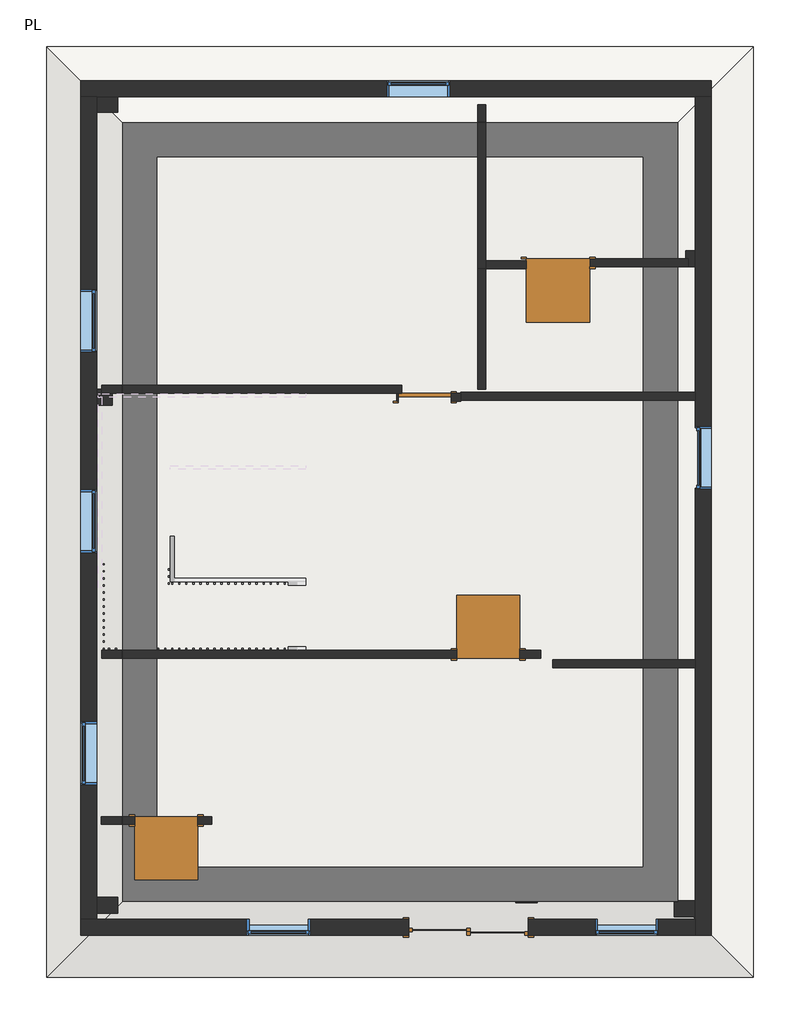
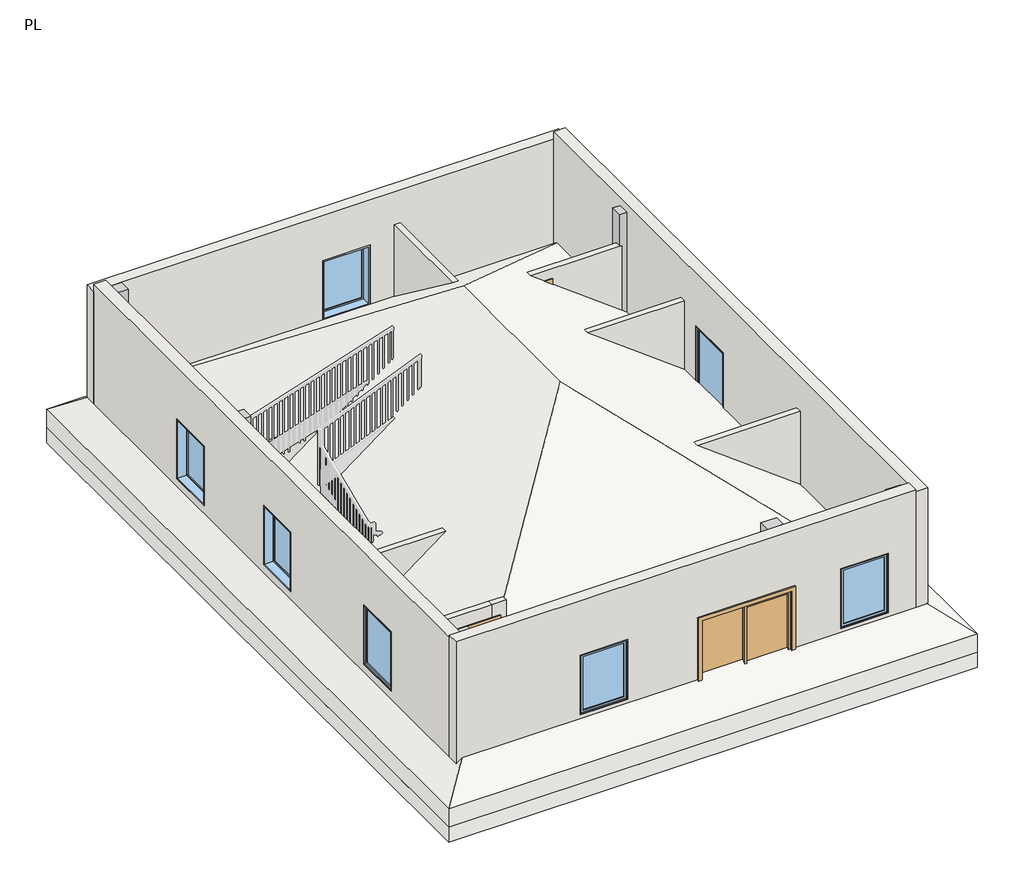
# One storey, part 1 of 3: 15 walls, 7 windows, 6 columns, 5 doors, 1 roof, 1 slab.
"""IFC4 building model written with IfcOpenShell, lengths in millimetres."""

from ifc_helpers import new_model, si_unit, frame, origin, origin_with_axes, place, context, project, spatial, polyline, outline, extrude, faceted_brep, transform, mapped, element, save
from components import door_ed3b37b7, door_0dbedf7e, door_f2b275c1, fixed_3_x_4_c1f32544

model = new_model("IFC4")

# Units and contexts
model_context = context("Model", 3, world=origin())
ifc_project = project(units=[si_unit("LENGTHUNIT", "METRE", prefix="MILLI")], contexts=[model_context])

# Site, building, storey
site = spatial("IfcSite", under=ifc_project)
building = spatial("IfcBuilding", under=site)
storey = spatial("IfcBuildingStorey", under=building, Name="PL", Elevation=0.0)

# Columns
placement = place(None, origin())
element("IfcColumn", 1, ObjectType="Rectangular Column : 1'9\"", at=placement, inside=storey, context=model_context, shape_type="SweptSolid", body=[
    extrude(outline(polyline([(10828.4334712, 491.3450307), (10828.4334712, 262.7450307), (10523.6334712, 262.7450307), (10523.6334712, 491.3450307), (10828.4334712, 491.3450307)])), origin_with_axes(), (0.0, 0.0, 1.0), 3048.0),
])
element("IfcColumn", 2, ObjectType="Rectangular Column : 1'9\"", at=placement, inside=storey, context=model_context, shape_type="SweptSolid", body=[
    extrude(outline(polyline([(8542.4334712, 694.5450307), (8542.4334712, 465.9450307), (8237.6334712, 465.9450307), (8237.6334712, 694.5450307), (8542.4334712, 694.5450307)])), origin_with_axes(), (0.0, 0.0, 1.0), 3048.0),
])
element("IfcColumn", 3, ObjectType="Rectangular Column : 1'9\"", at=placement, inside=storey, context=model_context, shape_type="SweptSolid", body=[
    extrude(outline(polyline([(2484.5334712, 542.1450307), (2484.5334712, 313.5450307), (2179.7334712, 313.5450307), (2179.7334712, 542.1450307), (2484.5334712, 542.1450307)])), origin_with_axes(), (0.0, 0.0, 1.0), 3048.0),
])
element("IfcColumn", 4, ObjectType="Rectangular Column : 1'9\"", at=placement, inside=storey, context=model_context, shape_type="Brep", body=[
    faceted_brep([(2408.3334712, 7654.1450307, 0.0), (2179.7334712, 7654.1450307, 0.0), (2179.7334712, 7882.7450307, 0.0), (2255.9334712, 7882.7450307, 0.0), (2255.9334712, 7825.5950307, 0.0), (2408.3334712, 7825.5950307, 0.0), (2408.3334712, 7882.7450307, 3048.0), (2408.3334712, 7654.1450307, 3048.0), (2408.3334712, 7825.5950307, 2213.5109209), (2408.3334712, 7882.7450307, 2213.5109209), (2179.7334712, 7654.1450307, 3048.0), (2179.7334712, 7882.7450307, 3048.0), (2255.9334712, 7882.7450307, 2213.5109209), (2255.9334712, 7825.5950307, 2213.5109209)], [[[0, 1, 2, 3, 4, 5]], [[6, 7, 0, 5, 8, 9]], [[0, 7, 10, 1]], [[11, 6, 9, 12, 3, 2]], [[7, 6, 11, 10]], [[2, 1, 10, 11]], [[4, 13, 8, 5]], [[8, 13, 12, 9]], [[13, 4, 3, 12]]]),
])
element("IfcColumn", 5, ObjectType="Rectangular Column : 1'9\"", at=placement, inside=storey, context=model_context, shape_type="SweptSolid", body=[
    extrude(outline(polyline([(2484.5334712, 12111.8450307), (2484.5334712, 11883.2450307), (2179.7334712, 11883.2450307), (2179.7334712, 12111.8450307), (2484.5334712, 12111.8450307)])), origin_with_axes(), (0.0, 0.0, 1.0), 3048.0),
])
element("IfcColumn", 6, ObjectType="Rectangular Column : 1'9\"", at=placement, inside=storey, context=model_context, shape_type="Brep", body=[
    faceted_brep([(10688.7334712, 9882.9950307, 0.0), (10828.4334712, 9882.9950307, 0.0), (10828.4334712, 9654.3950307, 0.0), (10726.8334712, 9654.3950307, 0.0), (10726.8334712, 9768.6950307, 0.0), (10688.7334712, 9768.6950307, 0.0), (10828.4334712, 9654.3950307, 3048.0), (10688.7334712, 9654.3950307, 3048.0), (10688.7334712, 9654.3950307, 2404.1722745), (10726.8334712, 9654.3950307, 2404.1722745), (10688.7334712, 9882.9950307, 3048.0), (10688.7334712, 9768.6950307, 2404.1722745), (10828.4334712, 9882.9950307, 3048.0), (10726.8334712, 9768.6950307, 2404.1722745)], [[[0, 1, 2, 3, 4, 5]], [[6, 7, 8, 9, 3, 2]], [[7, 10, 0, 5, 11, 8]], [[0, 10, 12, 1]], [[10, 7, 6, 12]], [[2, 1, 12, 6]], [[4, 13, 11, 5]], [[13, 4, 3, 9]], [[13, 9, 8, 11]]]),
])

# Doors
door_shape = door_ed3b37b7(model_context)
element("IfcDoor", 7, ObjectType="Door-Double-Sliding : 68\" x 80\"", at=placement, inside=storey, context=model_context, shape_type="MappedRepresentation", body=[
    mapped(door_shape, transform((7551.8334712, 237.3450307, 0.0), x_axis=(-1.0, 0.0, 0.0), y_axis=(0.0, -1.0, 0.0), z_axis=(0.0, 0.0, 1.0))),
])
door_2_shape = door_0dbedf7e(model_context)
element("IfcDoor", 8, ObjectType="Single-Flush : 2'8\"X7'", at=placement, inside=storey, context=model_context, shape_type="MappedRepresentation", body=[
    mapped(door_2_shape, transform((7837.5834712, 4053.6950307, 0.0), x_axis=(1.0, 0.0, 0.0), y_axis=(0.0, 1.0, 0.0), z_axis=(0.0, 0.0, 1.0))),
])
element("IfcDoor", 9, ObjectType="Single-Flush : 2'8\"X7'", at=placement, inside=storey, context=model_context, shape_type="MappedRepresentation", body=[
    mapped(door_2_shape, transform((3184.605209, 1653.3950307, 0.0), x_axis=(-1.0, 0.0, 0.0), y_axis=(0.0, -1.0, 0.0), z_axis=(0.0, 0.0, 1.0))),
])
element("IfcDoor", 10, ObjectType="Single-Flush : 2'8\"X7'", at=placement, inside=storey, context=model_context, shape_type="MappedRepresentation", body=[
    mapped(door_2_shape, transform((8847.2334712, 9711.5450307, 0.0), x_axis=(-1.0, 0.0, 0.0), y_axis=(0.0, -1.0, 0.0), z_axis=(0.0, 0.0, 1.0))),
])
door_3_shape = door_f2b275c1(model_context)
element("IfcDoor", 11, ObjectType="Single-Flush : 30\" x 80\"", at=placement, inside=storey, context=model_context, shape_type="MappedRepresentation", body=[
    mapped(door_3_shape, transform((6919.3734712, 7768.4450307, 0.0), x_axis=(-1.0, 0.0, 0.0), y_axis=(0.0, -1.0, 0.0), z_axis=(0.0, 0.0, 1.0))),
])

# Roof
element("IfcRoof", 12, ObjectType="Generic - 12\"", at=placement, inside=storey, context=model_context, shape_type="Brep", body=[
    faceted_brep([(11666.6334712, 12835.7450307, 0.0), (6561.2334712, 7730.3450307, 3829.05), (1455.8334712, 12835.7450307, 0.0), (6561.2334712, 4491.8450307, 3829.05), (1455.8334712, -613.5549693, 0.0), (11666.6334712, -613.5549693, 0.0), (11666.6334712, 12835.7450307, 381.0), (1455.8334712, 12835.7450307, 381.0), (6561.2334712, 7730.3450307, 4210.05), (1455.8334712, -613.5549693, 381.0), (6561.2334712, 4491.8450307, 4210.05), (11666.6334712, -613.5549693, 381.0)], [[[0, 1, 2]], [[2, 1, 3, 4]], [[4, 3, 5]], [[1, 0, 5, 3]], [[6, 7, 8]], [[7, 9, 10, 8]], [[9, 11, 10]], [[6, 8, 10, 11]], [[2, 7, 6, 0]], [[4, 9, 7, 2]], [[5, 11, 9, 4]], [[0, 6, 11, 5]]]),
])

# Slab
element("IfcSlab", 13, ObjectType="Generic - 12\"", at=placement, inside=storey, context=model_context, shape_type="SweptSolid", body=[
    extrude(outline(polyline([(11666.6334712, 12835.7450307), (11666.6334712, -613.5549693), (1455.8334712, -613.5549693), (1455.8334712, 12835.7450307), (11666.6334712, 12835.7450307)])), frame((0.0, 0.0, -304.8), z_axis=(0.0, 0.0, 1.0), x_axis=(1.0, 0.0, 0.0)), (0.0, 0.0, 1.0), 304.8),
])

# Walls
element("IfcWall", 14, ObjectType="Generic - 4.5\"", at=placement, inside=storey, context=model_context, shape_type="Brep", body=[
    faceted_brep([(7437.5334712, 7725.3187832, 0.0), (10828.4334712, 7725.3187832, 0.0), (10828.4334712, 7725.3187832, 2412.2250304), (7437.5334712, 7725.3187832, 2412.2250304), (7437.5334712, 7839.6187832, 0.0), (7437.5334712, 7839.6187832, 2412.2250304), (10828.4334712, 7839.6187832, 2412.2250304), (10828.4334712, 7839.6187832, 0.0), (7437.5334712, 7825.5950307, 0.0)], [[[0, 1, 2, 3]], [[4, 5, 6, 7]], [[1, 0, 8, 4, 7]], [[3, 2, 6, 5]], [[0, 3, 5, 4, 8]], [[2, 1, 7, 6]]]),
])
element("IfcWall", 15, ObjectType="Generic - 4.5\"", at=placement, inside=storey, context=model_context, shape_type="Brep", body=[
    faceted_brep([(7685.1834712, 11997.5450307, 0.0), (7685.1834712, 9628.9950307, 0.0), (7685.1834712, 9628.9950307, 2417.5045294), (7685.1834712, 9628.9950307, 2471.7996307), (7685.1834712, 11997.5450307, 2471.7996307), (7799.4834712, 11997.5450307, 0.0), (7799.4834712, 11997.5450307, 2471.7996307), (7799.4834712, 9628.9950307, 2471.7996307), (7799.4834712, 9628.9950307, 2435.357592), (7799.4834712, 9628.9950307, 2417.5045294), (7799.4834712, 9628.9950307, 0.0), (7799.4834712, 9743.2950307, 0.0)], [[[0, 1, 2, 3, 4]], [[5, 6, 7, 8, 9, 10, 11]], [[1, 0, 5, 11, 10]], [[4, 3, 7, 6]], [[0, 4, 6, 5]], [[1, 10, 9, 8, 7, 3, 2]]]),
])
element("IfcWall", 16, ObjectType="Generic - 4.5\"", at=placement, inside=storey, context=model_context, shape_type="SweptSolid", body=[
    extrude(outline(polyline([(7799.4834712, 9628.9950307), (7799.4834712, 7882.7450307), (7685.1834712, 7882.7450307), (7685.1834712, 9628.9950307), (7799.4834712, 9628.9950307)])), origin_with_axes(), (0.0, 0.0, 1.0), 2417.5045294),
])
element("IfcWall", 17, ObjectType="Generic - 4.5\"", at=placement, inside=storey, context=model_context, shape_type="SweptSolid", body=[
    extrude(outline(polyline([(8390.0334712, 9628.9950307), (7799.4834712, 9628.9950307), (7799.4834712, 9743.2950307), (8390.0334712, 9743.2950307), (8390.0334712, 9628.9950307)])), origin_with_axes(), (0.0, 0.0, 1.0), 2435.357592),
])
element("IfcWall", 18, ObjectType="Generic - 4.5\"", at=placement, inside=storey, context=model_context, shape_type="Brep", body=[
    faceted_brep([(10726.8334712, 9654.3950307, 0.0), (10726.8334712, 9654.3950307, 2404.1722745), (10688.7334712, 9654.3950307, 2404.1722745), (8390.0334712, 9654.3950307, 2404.1722745), (8390.0334712, 9654.3950307, 2133.6), (9304.4334712, 9654.3950307, 2133.6), (9304.4334712, 9654.3950307, 0.0), (10726.8334712, 9768.6950307, 2404.1722745), (10726.8334712, 9768.6950307, 0.0), (10688.7334712, 9768.6950307, 0.0), (9304.4334712, 9768.6950307, 0.0), (9304.4334712, 9768.6950307, 2133.6), (8390.0334712, 9768.6950307, 2133.6), (8390.0334712, 9768.6950307, 2404.1722745), (10688.7334712, 9768.6950307, 2404.1722745)], [[[0, 1, 2, 3, 4, 5, 6]], [[7, 8, 9, 10, 11, 12, 13, 14]], [[8, 0, 6, 10, 9]], [[1, 0, 8, 7]], [[3, 2, 1, 7, 14, 13]], [[3, 13, 12, 4]], [[11, 5, 4, 12]], [[5, 11, 10, 6]]]),
])
element("IfcWall", 19, ObjectType="Generic - 4.5\"", at=placement, inside=storey, context=model_context, shape_type="SweptSolid", body=[
    extrude(outline(polyline([(2467.0443884, 3565.605209), (2467.0443884, 2243.2334712), (0.0, 2243.2334712), (0.0, 2727.405209), (2133.6, 2727.405209), (2133.6, 3565.605209), (2467.0443884, 3565.605209)])), frame((0.0, 1596.2450307, 0.0), z_axis=(0.0, 1.0, 0.0), x_axis=(0.0, 0.0, 1.0)), (0.0, 0.0, 1.0), 114.3),
])
element("IfcWall", 20, ObjectType="Generic - 4.5\"", at=placement, inside=storey, context=model_context, shape_type="SweptSolid", body=[
    extrude(outline(polyline([(0.0, 3843.4334712), (2467.0443884, 3843.4334712), (2467.0443884, 3565.605209), (2133.6, 3565.605209), (2133.6, 3641.805209), (0.0, 3641.805209), (0.0, 3843.4334712)])), frame((0.0, 1596.2450307, 0.0), z_axis=(0.0, 1.0, 0.0), x_axis=(0.0, 0.0, 1.0)), (0.0, 0.0, 1.0), 114.3),
])
element("IfcWall", 21, ObjectType="Generic - 4.5\"", at=placement, inside=storey, context=model_context, shape_type="SweptSolid", body=[
    extrude(outline(polyline([(2133.6, 8294.7834712), (0.0, 8294.7834712), (0.0, 8599.5834712), (2337.0025818, 8599.5834712), (2337.0025818, 2255.9334712), (0.0, 2255.9334712), (0.0, 7380.3834712), (2133.6, 7380.3834712), (2133.6, 8294.7834712)])), frame((0.0, 3996.5450307, 0.0), z_axis=(0.0, 1.0, 0.0), x_axis=(0.0, 0.0, 1.0)), (0.0, 0.0, 1.0), 114.3),
])
element("IfcWall", 22, ObjectType="Generic - 4.5\"", at=placement, inside=storey, context=model_context, shape_type="Brep", body=[
    faceted_brep([(6512.9734712, 7711.2950307, 0.0), (6538.3734712, 7711.2950307, 0.0), (6538.3734712, 7711.2950307, 2032.0), (7300.3734712, 7711.2950307, 2032.0), (7300.3734712, 7711.2950307, 0.0), (7437.5334712, 7711.2950307, 0.0), (7437.5334712, 7711.2950307, 2334.4745508), (6512.9734712, 7711.2950307, 2334.4745508), (6538.3734712, 7825.5950307, 2032.0), (6538.3734712, 7825.5950307, 0.0), (6512.9734712, 7825.5950307, 0.0), (6512.9734712, 7825.5950307, 2334.4745508), (7437.5334712, 7825.5950307, 2334.4745508), (7437.5334712, 7825.5950307, 0.0), (7300.3734712, 7825.5950307, 0.0), (7300.3734712, 7825.5950307, 2032.0), (7437.5334712, 7725.3187832, 0.0)], [[[0, 1, 2, 3, 4, 5, 6, 7]], [[8, 9, 10, 11, 12, 13, 14, 15]], [[14, 13, 16, 5, 4]], [[10, 9, 1, 0]], [[6, 5, 16, 13, 12]], [[7, 6, 12, 11]], [[0, 7, 11, 10]], [[2, 1, 9, 8]], [[3, 2, 8, 15]], [[4, 3, 15, 14]]]),
])
element("IfcWall", 23, ObjectType="Generic - 4.5\"", at=placement, inside=storey, context=model_context, shape_type="SweptSolid", body=[
    extrude(outline(polyline([(10828.4334712, 3860.0200307), (8771.0334712, 3860.0200307), (8771.0334712, 3974.3200307), (10828.4334712, 3974.3200307), (10828.4334712, 3860.0200307)])), origin_with_axes(), (0.0, 0.0, 1.0), 2500.2242251),
])
element("IfcWall", 24, ObjectType="Generic - 4.5\"", at=placement, inside=storey, context=model_context, shape_type="Brep", body=[
    faceted_brep([(2255.9334712, 7825.5950307, 0.0), (2408.3334712, 7825.5950307, 0.0), (6589.1734712, 7825.5950307, 0.0), (6589.1734712, 7825.5950307, 2213.5109209), (2408.3334712, 7825.5950307, 2213.5109209), (2255.9334712, 7825.5950307, 2213.5109209), (2255.9334712, 7939.8950307, 0.0), (2255.9334712, 7939.8950307, 2213.5109209), (6589.1734712, 7939.8950307, 2213.5109209), (6589.1734712, 7939.8950307, 0.0), (2255.9334712, 7882.7450307, 0.0), (2255.9334712, 7882.7450307, 2213.5109209)], [[[0, 1, 2, 3, 4, 5]], [[6, 7, 8, 9]], [[2, 1, 0, 10, 6, 9]], [[3, 2, 9, 8]], [[5, 4, 3, 8, 7, 11]], [[0, 5, 11, 7, 6, 10]]]),
])
element("IfcWall", 25, ObjectType="Generic -9\"", at=placement, inside=storey, context=model_context, shape_type="Brep", body=[
    faceted_brep([(1951.1334712, 12111.8450307, 0.0), (2179.7334712, 12111.8450307, 0.0), (2484.5334712, 12111.8450307, 0.0), (10828.4334712, 12111.8450307, 0.0), (11057.0334712, 12111.8450307, 0.0), (11057.0334712, 12111.8450307, 3048.0), (2484.5334712, 12111.8450307, 3048.0), (2179.7334712, 12111.8450307, 3048.0), (1951.1334712, 12111.8450307, 3048.0), (7285.1334712, 12111.8450307, 2133.6), (7285.1334712, 12111.8450307, 914.4), (6370.7334712, 12111.8450307, 914.4), (6370.7334712, 12111.8450307, 2133.6), (1951.1334712, 12340.4450307, 0.0), (1951.1334712, 12340.4450307, 3048.0), (11057.0334712, 12340.4450307, 3048.0), (11057.0334712, 12340.4450307, 0.0), (7285.1334712, 12340.4450307, 2133.6), (6370.7334712, 12340.4450307, 2133.6), (6370.7334712, 12340.4450307, 914.4), (7285.1334712, 12340.4450307, 914.4)], [[[0, 1, 2, 3, 4, 5, 6, 7, 8], [9, 10, 11, 12]], [[13, 14, 15, 16], [17, 18, 19, 20]], [[4, 3, 2, 1, 0, 13, 16]], [[8, 7, 6, 5, 15, 14]], [[5, 4, 16, 15]], [[0, 8, 14, 13]], [[10, 9, 17, 20]], [[11, 10, 20, 19]], [[12, 11, 19, 18]], [[9, 12, 18, 17]]]),
])
element("IfcWall", 26, ObjectType="Generic -9\"", at=placement, inside=storey, context=model_context, shape_type="Brep", body=[
    faceted_brep([(10828.4334712, 12111.8450307, 0.0), (10828.4334712, 9882.9950307, 0.0), (10828.4334712, 9654.3950307, 0.0), (10828.4334712, 7839.6187832, 0.0), (10828.4334712, 7725.3187832, 0.0), (10828.4334712, 3974.3200307, 0.0), (10828.4334712, 3860.0200307, 0.0), (10828.4334712, 491.3450307, 0.0), (10828.4334712, 262.7450307, 0.0), (10828.4334712, 224.6450307, 0.0), (10828.4334712, -3.9549693, 0.0), (10828.4334712, -3.9549693, 3200.4), (10828.4334712, 12111.8450307, 3200.4), (10828.4334712, 7350.6687832, 2133.6), (10828.4334712, 6436.2687832, 2133.6), (10828.4334712, 6436.2687832, 914.4), (10828.4334712, 7350.6687832, 914.4), (11057.0334712, 12111.8450307, 0.0), (11057.0334712, 12111.8450307, 3048.0), (11057.0334712, 12111.8450307, 3200.4), (11057.0334712, -3.9549693, 3200.4), (11057.0334712, -3.9549693, 0.0), (11057.0334712, 7350.6687832, 2133.6), (11057.0334712, 7350.6687832, 914.4), (11057.0334712, 6436.2687832, 914.4), (11057.0334712, 6436.2687832, 2133.6)], [[[0, 1, 2, 3, 4, 5, 6, 7, 8, 9, 10, 11, 12], [13, 14, 15, 16]], [[17, 18, 19, 20, 21], [22, 23, 24, 25]], [[10, 9, 8, 7, 6, 5, 4, 3, 2, 1, 0, 17, 21]], [[12, 11, 20, 19]], [[0, 12, 19, 18, 17]], [[11, 10, 21, 20]], [[23, 22, 13, 16]], [[24, 23, 16, 15]], [[25, 24, 15, 14]], [[22, 25, 14, 13]]]),
])
element("IfcWall", 27, ObjectType="Generic -9\"", at=placement, inside=storey, context=model_context, shape_type="Brep", body=[
    faceted_brep([(6688.2334712, 224.6450307, 2032.0), (6688.2334712, 224.6450307, 0.0), (2179.7334712, 224.6450307, 0.0), (1951.1334712, 224.6450307, 0.0), (1951.1334712, 224.6450307, 3200.4), (1951.1334712, 224.6450307, 3244.9103785), (10828.4334712, 224.6450307, 3244.9103785), (10828.4334712, 224.6450307, 0.0), (8415.4334712, 224.6450307, 0.0), (8415.4334712, 224.6450307, 2032.0), (4351.4334712, 224.6450307, 2133.6), (4351.4334712, 224.6450307, 914.4), (5265.8334712, 224.6450307, 914.4), (5265.8334712, 224.6450307, 2133.6), (9380.6334712, 224.6450307, 2133.6), (9380.6334712, 224.6450307, 914.4), (10295.0334712, 224.6450307, 914.4), (10295.0334712, 224.6450307, 2133.6), (1951.1334712, -3.9549693, 0.0), (6688.2334712, -3.9549693, 0.0), (6688.2334712, -3.9549693, 2032.0), (8415.4334712, -3.9549693, 2032.0), (8415.4334712, -3.9549693, 0.0), (10828.4334712, -3.9549693, 0.0), (10828.4334712, -3.9549693, 3200.4), (10828.4334712, -3.9549693, 3244.9103785), (1951.1334712, -3.9549693, 3244.9103785), (4351.4334712, -3.9549693, 2133.6), (5265.8334712, -3.9549693, 2133.6), (5265.8334712, -3.9549693, 914.4), (4351.4334712, -3.9549693, 914.4), (9380.6334712, -3.9549693, 2133.6), (10295.0334712, -3.9549693, 2133.6), (10295.0334712, -3.9549693, 914.4), (9380.6334712, -3.9549693, 914.4)], [[[0, 1, 2, 3, 4, 5, 6, 7, 8, 9], [10, 11, 12, 13], [14, 15, 16, 17]], [[18, 19, 20, 21, 22, 23, 24, 25, 26], [27, 28, 29, 30], [31, 32, 33, 34]], [[8, 7, 23, 22]], [[3, 2, 1, 19, 18]], [[6, 5, 26, 25]], [[7, 6, 25, 24, 23]], [[5, 4, 3, 18, 26]], [[11, 10, 27, 30]], [[12, 11, 30, 29]], [[13, 12, 29, 28]], [[10, 13, 28, 27]], [[15, 14, 31, 34]], [[16, 15, 34, 33]], [[17, 16, 33, 32]], [[14, 17, 32, 31]], [[22, 21, 9, 8]], [[20, 19, 1, 0]], [[21, 20, 0, 9]]]),
])
element("IfcWall", 28, ObjectType="Generic -9\"", at=placement, inside=storey, context=model_context, shape_type="Brep", body=[
    faceted_brep([(2179.7334712, 224.6450307, 0.0), (2179.7334712, 313.5450307, 0.0), (2179.7334712, 542.1450307, 0.0), (2179.7334712, 7654.1450307, 0.0), (2179.7334712, 7882.7450307, 0.0), (2179.7334712, 11883.2450307, 0.0), (2179.7334712, 12111.8450307, 0.0), (2179.7334712, 12111.8450307, 3048.0), (2179.7334712, 12111.8450307, 3200.4), (2179.7334712, 224.6450307, 3200.4), (2179.7334712, 8416.1450307, 2133.6), (2179.7334712, 9330.5450307, 2133.6), (2179.7334712, 9330.5450307, 914.4), (2179.7334712, 8416.1450307, 914.4), (2179.7334712, 5520.5450307, 2133.6), (2179.7334712, 6434.9450307, 2133.6), (2179.7334712, 6434.9450307, 914.4), (2179.7334712, 5520.5450307, 914.4), (2179.7334712, 3082.1450307, 2133.6), (2179.7334712, 3082.1450307, 914.4), (2179.7334712, 2167.7450307, 914.4), (2179.7334712, 2167.7450307, 2133.6), (1951.1334712, 224.6450307, 0.0), (1951.1334712, 224.6450307, 3200.4), (1951.1334712, 12111.8450307, 3200.4), (1951.1334712, 12111.8450307, 3048.0), (1951.1334712, 12111.8450307, 0.0), (1951.1334712, 8416.1450307, 2133.6), (1951.1334712, 8416.1450307, 914.4), (1951.1334712, 9330.5450307, 914.4), (1951.1334712, 9330.5450307, 2133.6), (1951.1334712, 5520.5450307, 2133.6), (1951.1334712, 5520.5450307, 914.4), (1951.1334712, 6434.9450307, 914.4), (1951.1334712, 6434.9450307, 2133.6), (1951.1334712, 3082.1450307, 2133.6), (1951.1334712, 2167.7450307, 2133.6), (1951.1334712, 2167.7450307, 914.4), (1951.1334712, 3082.1450307, 914.4)], [[[0, 1, 2, 3, 4, 5, 6, 7, 8, 9], [10, 11, 12, 13], [14, 15, 16, 17], [18, 19, 20, 21]], [[22, 23, 24, 25, 26], [27, 28, 29, 30], [31, 32, 33, 34], [35, 36, 37, 38]], [[6, 5, 4, 3, 2, 1, 0, 22, 26]], [[9, 8, 24, 23]], [[8, 7, 6, 26, 25, 24]], [[0, 9, 23, 22]], [[28, 27, 10, 13]], [[29, 28, 13, 12]], [[30, 29, 12, 11]], [[27, 30, 11, 10]], [[32, 31, 14, 17]], [[33, 32, 17, 16]], [[34, 33, 16, 15]], [[31, 34, 15, 14]], [[19, 18, 35, 38]], [[20, 19, 38, 37]], [[21, 20, 37, 36]], [[18, 21, 36, 35]]]),
])

# Windows
fixed_3_x_4_shape = fixed_3_x_4_c1f32544(model_context)
element("IfcWindow", 29, ObjectType="Fixed : 3'x 4'", at=placement, inside=storey, context=model_context, shape_type="MappedRepresentation", body=[
    mapped(fixed_3_x_4_shape, transform((4770.5334712, 110.3450307, 0.0), x_axis=(-1.0, 0.0, 0.0), y_axis=(0.0, -1.0, 0.0), z_axis=(0.0, 0.0, 1.0))),
])
element("IfcWindow", 30, ObjectType="Fixed : 3'x 4'", at=placement, inside=storey, context=model_context, shape_type="MappedRepresentation", body=[
    mapped(fixed_3_x_4_shape, transform((10942.7334712, 6931.5687832, 0.0), x_axis=(0.0, 1.0, 0.0), y_axis=(-1.0, 0.0, 0.0), z_axis=(0.0, 0.0, 1.0))),
])
element("IfcWindow", 31, ObjectType="Fixed : 3'x 4'", at=placement, inside=storey, context=model_context, shape_type="MappedRepresentation", body=[
    mapped(fixed_3_x_4_shape, transform((6866.0334712, 12226.1450307, 0.0), x_axis=(1.0, 0.0, 0.0), y_axis=(0.0, 1.0, 0.0), z_axis=(0.0, 0.0, 1.0))),
])
element("IfcWindow", 32, ObjectType="Fixed : 3'x 4'", at=placement, inside=storey, context=model_context, shape_type="MappedRepresentation", body=[
    mapped(fixed_3_x_4_shape, transform((2065.4334712, 8835.2450307, 0.0), x_axis=(0.0, -1.0, 0.0), y_axis=(1.0, 0.0, 0.0), z_axis=(0.0, 0.0, 1.0))),
])
element("IfcWindow", 33, ObjectType="Fixed : 3'x 4'", at=placement, inside=storey, context=model_context, shape_type="MappedRepresentation", body=[
    mapped(fixed_3_x_4_shape, transform((2065.4334712, 5939.6450307, 0.0), x_axis=(0.0, -1.0, 0.0), y_axis=(1.0, 0.0, 0.0), z_axis=(0.0, 0.0, 1.0))),
])
element("IfcWindow", 34, ObjectType="Fixed : 3'x 4'", at=placement, inside=storey, context=model_context, shape_type="MappedRepresentation", body=[
    mapped(fixed_3_x_4_shape, transform((2065.4334712, 2663.0450307, 0.0), x_axis=(0.0, 1.0, 0.0), y_axis=(-1.0, 0.0, 0.0), z_axis=(0.0, 0.0, 1.0))),
])
element("IfcWindow", 35, ObjectType="Fixed : 3'x 4'", at=placement, inside=storey, context=model_context, shape_type="MappedRepresentation", body=[
    mapped(fixed_3_x_4_shape, transform((9799.7334712, 110.3450307, 0.0), x_axis=(-1.0, 0.0, 0.0), y_axis=(0.0, -1.0, 0.0), z_axis=(0.0, 0.0, 1.0))),
])

save(model, "model.ifc")

# Revit data of these elements
# Type "Rectangular Column : 1'9\""
#   Assembly Code = "B1010200"
#   Depth = 0' - 9"
#   Offset Base = 0' - 0"
#   Offset Top = 0' - 0"
#   Width = 1' - 0"
#   Material = none
# Type "Door-Double-Sliding : 68\" x 80\""
#   Type Mark = "10"
#   Construction Type Id = "opn-d45"
#   Assembly Code = "C1020"
#   Analytic Construction = "Wood frame, double glass door "
#   Thickness = 0' - 2"
#   Thermal Resistance (R) = 1.8150 (h·ft²·°F)/BTU
#   Heat Transfer Coefficient (U) = 0.5510 BTU/(h·ft²·°F)
#   Height = 6' - 8"
#   Rail Width = 0' - 2"
#   Stiles = 0' - 2"
#   Trim Projection Ext = 0' - 1"
#   Trim Projection Int = 0' - 1"
#   Trim Width = 0' - 3"
#   Width = 5' - 8"
#   Define Thermal Properties by = 1
#   Glazing = Glass
#   Panel Material = Wood - Birch - Solid Stained Light Low Gloss
#   Trim Material = Paint - Sienna
#   Visual Light Transmittance = 0
#   Solar Heat Gain Coefficient = 0
#   Function = (empty or 0)
#   Wall Closure = (empty or 0)
# Type "Single-Flush : 2'8\"X7'"
#   Type Mark = "8"
#   Construction Type Id = "MDOOR"
#   Assembly Code = "C1020"
#   Analytic Construction = "Metal"
#   Thickness = 3' - 0"
#   Heat Transfer Coefficient (U) = 0.651978 BTU/(h·ft²·°F)
#   Height = 7' - 0"
#   Trim Projection Ext = 0' - 1"
#   Trim Projection Int = 0' - 1"
#   Trim Width = 0' - 3"
#   Width = 3' - 0"
#   Define Thermal Properties by = 1
#   Door Material = Door - Panel
#   Frame Material = Door - Frame
#   Visual Light Transmittance = 0
#   Solar Heat Gain Coefficient = 0
#   Function = (empty or 0)
#   Wall Closure = (empty or 0)
# Type "Single-Flush : 30\" x 80\""
#   Type Mark = "5"
#   Construction Type Id = "MDOOR"
#   Assembly Code = "C1020"
#   Analytic Construction = "Metal"
#   Thickness = 0' - 2"
#   Heat Transfer Coefficient (U) = 0.651978 BTU/(h·ft²·°F)
#   Height = 6' - 8"
#   Trim Projection Ext = 0' - 1"
#   Trim Projection Int = 0' - 1"
#   Trim Width = 0' - 3"
#   Width = 2' - 6"
#   Define Thermal Properties by = 1
#   Define Thermal Properties by = 1
#   Door Material = Door - Panel
#   Frame Material = Door - Frame
#   Visual Light Transmittance = 0
#   Solar Heat Gain Coefficient = 0
#   Function = (empty or 0)
#   Wall Closure = (empty or 0)
# Type "Generic - 12\""
#   Assembly Code = "B1020"
#   Layers, outside or top first: 1' - 0" no material (function 1)
# Type "Generic - 12\""
#   Assembly Code = "B1010"
#   Function = 0
#   Layers, outside or top first: 1' - 0" no material (function 1)
# Type "Generic - 4.5\""
#   Assembly Code = "B2010"
#   Layers, outside or top first: 0' - 4 1/2" no material (function 1)
# Type "Generic -9\""
#   Assembly Code = "B2010"
#   Layers, outside or top first: 0' - 9" no material (function 1)
# Type "Fixed : 3'x 4'"
#   Type Mark = "18"
#   Construction Type Id = "GSP4R"
#   Assembly Code = "B2020100"
#   Analytic Construction = "1/8 in Pilkington single glazing"
#   Visual Light Transmittance = 0.9
#   Solar Heat Gain Coefficient = 0.78
#   Heat Transfer Coefficient (U) = 0.6496 BTU/(h·ft²·°F)
#   Height = 4' - 0"
#   Default Sill Height = 3' - 0"
#   Width = 3' - 0"
#   Window Inset = 0' - 0 3/4"
#   Define Thermal Properties by = 1
#   Glass Pane Material = Glass
#   Sash Material = Sash
#   Wall Closure = (empty or 0)
# Elements 1, 3, 4, 5, 6 (IfcColumn, "Rectangular Column : 1'9\"")
#   Phase Created = New Construction
#   Materials on its faces: "Default Wall"
# Element 2 (IfcColumn, "Rectangular Column : 1'9\"")
#   Phase Created = New Construction
# Element 7 (IfcDoor, "Door-Double-Sliding : 68\" x 80\"")
#   Phase Created = New Construction
#   Materials on its faces: "Paint - Sienna", "Wood - Birch - Solid Stained Light Low Gloss", "Glass"
# Elements 8, 9, 10 (IfcDoor, "Single-Flush : 2'8\"X7'")
#   Phase Created = New Construction
#   Materials on its faces: "Door - Frame", "Door - Panel"
# Element 11 (IfcDoor, "Single-Flush : 30\" x 80\"")
#   Phase Created = New Construction
#   Materials on its faces: "Door - Frame", "Door - Panel"
# Element 12 (IfcRoof, "Generic - 12\"")
#   built-in parameter 1001705 = 13.8125 (stored number, unit not read)
#   built-in parameter 1001710 = 33615
#   Phase Created = New Construction
#   Materials on its faces: "Default Roof"
# Element 13 (IfcSlab, "Generic - 12\"")
#   Height Offset From Level = 0' - 0"
#   Phase Created = New Construction
#   Materials on its faces: "Default Floor"
# Element 14 (IfcWall, "Generic - 4.5\"")
#   Top Offset = 1' - 10.96949"
#   Base Offset = 0' - 0"
#   Unconnected Height = 7' - 10.96949"
#   wall height = 7' - 10.96949"
#   Phase Created = New Construction
#   Base Constraint = PL
#   Materials on its faces: "Default Wall"
# Element 15 (IfcWall, "Generic - 4.5\"")
#   Top Offset = 2' - 1.31495"
#   Base Offset = 0' - 0"
#   Unconnected Height = 8' - 1.31495"
#   wall height = 8' - 1.31495"
#   Phase Created = New Construction
#   Base Constraint = PL
#   Materials on its faces: "Default Wall"
# Element 16 (IfcWall, "Generic - 4.5\"")
#   Top Offset = 1' - 11.17734"
#   Base Offset = 0' - 0"
#   Unconnected Height = 7' - 11.17734"
#   wall height = 7' - 11.17734"
#   Phase Created = New Construction
#   Base Constraint = PL
#   Materials on its faces: "Default Wall"
# Element 17 (IfcWall, "Generic - 4.5\"")
#   Top Offset = 1' - 11.88022"
#   Base Offset = 0' - 0"
#   Unconnected Height = 7' - 11.88022"
#   wall height = 7' - 11.88022"
#   Phase Created = New Construction
#   Base Constraint = PL
#   Materials on its faces: "Default Wall"
# Element 18 (IfcWall, "Generic - 4.5\"")
#   Top Offset = 1' - 10.65245"
#   Base Offset = 0' - 0"
#   Unconnected Height = 7' - 10.65245"
#   wall height = 7' - 10.65245"
#   Phase Created = New Construction
#   Base Constraint = PL
#   Materials on its faces: "Default Wall"
# Elements 19, 20 (IfcWall, "Generic - 4.5\"")
#   Top Offset = 2' - 1.12773"
#   Base Offset = 0' - 0"
#   Unconnected Height = 8' - 1.12773"
#   wall height = 8' - 1.12773"
#   Phase Created = New Construction
#   Base Constraint = PL
#   Materials on its faces: "Default Wall"
# Element 21 (IfcWall, "Generic - 4.5\"")
#   Top Offset = 1' - 8.00798"
#   Base Offset = 0' - 0"
#   Unconnected Height = 7' - 8.00798"
#   wall height = 7' - 8.00798"
#   Phase Created = New Construction
#   Base Constraint = PL
#   Materials on its faces: "Default Wall"
# Element 22 (IfcWall, "Generic - 4.5\"")
#   Top Offset = 1' - 7.90845"
#   Base Offset = 0' - 0"
#   Unconnected Height = 7' - 7.90845"
#   wall height = 7' - 7.90845"
#   Phase Created = New Construction
#   Base Constraint = PL
#   Materials on its faces: "Default Wall"
# Element 23 (IfcWall, "Generic - 4.5\"")
#   Top Offset = 2' - 2.43402"
#   Base Offset = 0' - 0"
#   Unconnected Height = 8' - 2.43402"
#   wall height = 8' - 2.43402"
#   Phase Created = New Construction
#   Base Constraint = PL
#   Materials on its faces: "Default Wall"
# Element 24 (IfcWall, "Generic - 4.5\"")
#   Top Offset = 1' - 3.1461"
#   Base Offset = 0' - 0"
#   Unconnected Height = 7' - 3.1461"
#   wall height = 7' - 3.1461"
#   Phase Created = New Construction
#   Base Constraint = PL
#   Materials on its faces: "Default Wall"
# Element 25 (IfcWall, "Generic -9\"")
#   Top Offset = 4' - 0"
#   Base Offset = 0' - 0"
#   Unconnected Height = 10' - 0"
#   wall height = 10' - 0"
#   Phase Created = New Construction
#   Base Constraint = PL
#   Materials on its faces: "Default Wall"
# Elements 26, 28 (IfcWall, "Generic -9\"")
#   Top Offset = 0' - 0"
#   Base Offset = 0' - 0"
#   Unconnected Height = 10' - 6"
#   wall height = 10' - 6"
#   Phase Created = New Construction
#   Base Constraint = PL
#   Materials on its faces: "Default Wall"
# Element 27 (IfcWall, "Generic -9\"")
#   Top Offset = 4' - 7.75238"
#   Base Offset = 0' - 0"
#   Unconnected Height = 10' - 7.75238"
#   wall height = 10' - 7.75238"
#   Phase Created = New Construction
#   Base Constraint = PL
#   Materials on its faces: "Default Wall"
# Element 29 (IfcWindow, "Fixed : 3'x 4'")
#   Mark = "16"
#   Phase Created = New Construction
#   Materials on its faces: "Sash", "Glass"
# Element 30 (IfcWindow, "Fixed : 3'x 4'")
#   Mark = "17"
#   Phase Created = New Construction
#   Materials on its faces: "Sash", "Glass"
# Element 31 (IfcWindow, "Fixed : 3'x 4'")
#   Mark = "18"
#   Phase Created = New Construction
#   Materials on its faces: "Sash", "Glass"
# Element 32 (IfcWindow, "Fixed : 3'x 4'")
#   Mark = "19"
#   Phase Created = New Construction
#   Materials on its faces: "Sash", "Glass"
# Element 33 (IfcWindow, "Fixed : 3'x 4'")
#   Mark = "20"
#   Phase Created = New Construction
#   Materials on its faces: "Sash", "Glass"
# Element 34 (IfcWindow, "Fixed : 3'x 4'")
#   Mark = "21"
#   Phase Created = New Construction
#   Materials on its faces: "Sash", "Glass"
# Element 35 (IfcWindow, "Fixed : 3'x 4'")
#   Mark = "22"
#   Phase Created = New Construction
#   Materials on its faces: "Sash", "Glass"
# Materials
#   "Glass": class "Glass", colour RGB 0 128 192, transparency 0.75, Description = "Soda Lime Glass", Cost = 0
#   "Wood - Birch - Solid Stained Light Low Gloss": class "Wood", colour RGB 210 159 95, transparency 0, Cost = 0
#   "Paint - Sienna": colour RGB 118 70 51, transparency 0, Cost = 0
#   "Door - Panel": class "Wood", colour RGB 210 159 95, transparency 0, Cost = 0
#   "Door - Frame": colour RGB 118 70 51, transparency 0, Cost = 0
#   "Sash": class "Wood", colour RGB 224 178 126, transparency 0, Cost = 0
#   "Default Wall": colour RGB 128 128 128, transparency 0, Cost = 0
#   "Default Roof": colour RGB 88 101 114, transparency 0, Cost = 0
#   "Default Floor": colour RGB 128 128 128, transparency 0, Cost = 0
